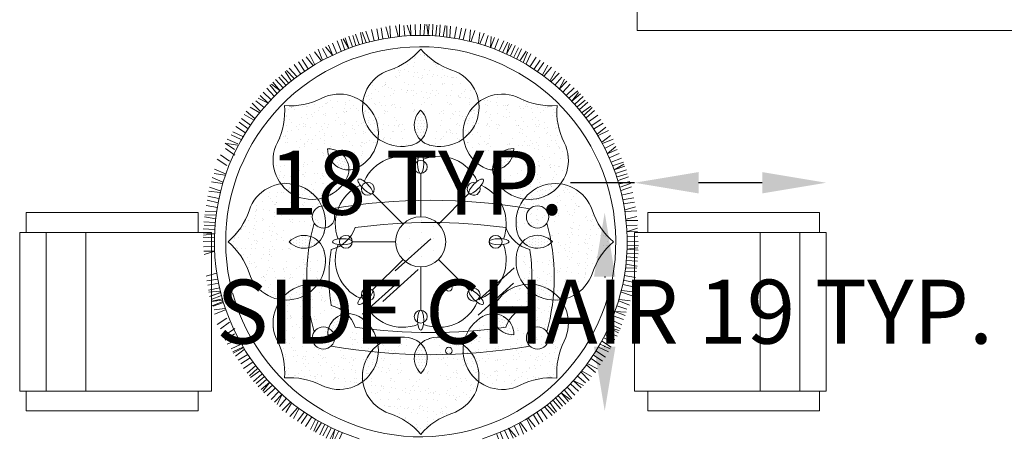
# Model space of a CAD drawing. Units: inches. Extents: x 1994 to 3075, y 3517 to 3950.
# Tile 56 of 58: x 2927 to 3019, y 3698 to 3737. Entities that reach past the tile are written whole.
import ezdxf

# ---------------------------------------------------------------- set-up
doc = ezdxf.new("R2010")
doc.units = ezdxf.units.IN
for name, color, linetype, lineweight in [('A-ANNO-DIMS', 2, 'Continuous', 18), ('A-FLOR-CASE', 8, 'Continuous', 18), ('A-FURN', 8, 'Continuous', 18), ('A-FURN-PATT', 8, 'Continuous', 13)]:
    doc.layers.add(name, color=color, linetype=linetype, lineweight=lineweight)
doc.styles.get("Standard").update_dxf_attribs({"font": 'arial.ttf'})
doc.dimstyles.get("Standard").update_dxf_attribs({"dimtxt": 6, "dimasz": 6, "dimexe": 0.18, "dimexo": 0.0625, "dimgap": 0.09, "dimtad": 0, "dimtih": 1, "dimtoh": 1, "dimdec": 4, "dimzin": 0, "dimdsep": 46, "dimlunit": 4, "dimtxsty": 'Standard', "dimcen": 0.09, "dimse1": 1, "dimse2": 1, "dimadec": 0, "dimazin": 0, "dimtfac": 1, "dimtdec": 4, "dimtofl": 0, "dimtmove": 0, "dimatfit": 3, "dimfxl": 1, "dimtolj": 1, "dimtzin": 0, "dimarcsym": 0})

# ---------------------------------------------------------------- blocks, each defined once
blk = doc.blocks.new('CHAIR-SIDE')
for p, q in [((0.619, 18.584), (16.725, 18.584)), ((0.619, 16.725), (0.619, 18.584)), ((16.725, 18.584), (16.725, 16.725)), ((0, 1.858), (0, 16.725)), ((0, 16.725), (17.964, 16.725)), ((2.478, 1.858), (2.478, 16.725)), ((6.195, 16.725), (6.195, 1.858)), ((17.964, 16.725), (17.964, 1.858)), ((17.964, 1.858), (0, 1.858)), ((0.619, 0), (0.619, 1.858)), ((16.725, 1.858), (16.725, 0)), ((16.725, 0), (0.619, 0))]:
    blk.add_line(p, q)
blk = doc.blocks.new('*D27')
at = {"layer": 'A-ANNO-DIMS', "color": 0, "lineweight": -2, "transparency": 16777216}
for p, q in [((2981.575, 3712.965), (2981.575, 3712.865)), ((2981.575, 3706.381), (2981.575, 3706.481))]:
    blk.add_line(p, q, dxfattribs=at)
at = {"layer": 'A-ANNO-DIMS', "color": 0, "transparency": 16777216}
for points in [[(2980.575, 3712.965), (2982.575, 3712.965), (2981.575, 3718.965)], [(2980.575, 3706.381), (2982.575, 3706.381), (2981.575, 3700.381)]]:
    blk.add_solid(points, dxfattribs=at)
at = {"layer": 'Defpoints', "color": 0, "transparency": 16777216}
for p in [(2984.363, 3718.965), (2981.575, 3700.381), (2984.363, 3700.381)]:
    blk.add_point(p, dxfattribs=at)
at = {"layer": 'A-ANNO-DIMS', "color": 0, "transparency": 16777216, "insert": (2981.575, 3709.673), "char_height": 6, "attachment_point": 5}
blk.add_mtext('\\A1;SIDE CHAIR 19 TYP.', dxfattribs=at)
blk = doc.blocks.new('*D28')
at = {"layer": 'A-ANNO-DIMS', "color": 0, "lineweight": -2, "transparency": 16777216}
for p, q in [((2984.363, 3721.752), (2978.363, 3721.752)), ((2996.327, 3721.752), (2990.363, 3721.752))]:
    blk.add_line(p, q, dxfattribs=at)
at = {"layer": 'A-ANNO-DIMS', "color": 0, "transparency": 16777216}
for points in [[(2990.363, 3722.752), (2990.363, 3720.752), (2984.363, 3721.752)], [(2996.327, 3722.752), (2996.327, 3720.752), (3002.327, 3721.752)]]:
    blk.add_solid(points, dxfattribs=at)
at = {"layer": 'Defpoints', "color": 0, "transparency": 16777216}
for p in [(2984.363, 3721.752), (2984.363, 3718.965), (3002.327, 3718.965)]:
    blk.add_point(p, dxfattribs=at)
at = {"layer": 'A-ANNO-DIMS', "color": 0, "transparency": 16777216, "insert": (2963.952, 3721.752), "char_height": 6, "attachment_point": 5}
blk.add_mtext('\\A1;18 TYP.', dxfattribs=at)

msp = doc.modelspace()

# ---------------------------------------------------------------- hatches: boundary and pattern name
at = {"layer": 'A-FURN-PATT'}
h = msp.add_hatch(dxfattribs=at)
h.set_pattern_fill('AR-SAND', color=256, scale=0.026605, angle=360, style=0)
h.set_pattern_definition([(142.5, (5370.1894, -656.1987), (0.04256891, 1.30208636), [0, -1.02716777, 0, -1.14880606, 0, -1.09812344]), (172.5, (5370.1894, -656.1987), (-1.19595894, 1.90711676), [0, -0.55412998, 0, -0.92580253, 0, -0.35477834]), (212.5, (5371.0206, -656.1987), (-2.10443915, 0.00382364), [0, -0.33788413, 0, -1.21638288, 0, -1.58805543]), (222.5, (5371.0206, -656.1987), (-2.03144575, 0.5931046), [0, -0.16894207, 0, -0.79740656, 0, -0.91228716])])
edge = h.paths.add_edge_path()
edge.add_arc((2962.5504, 3728.8135), 3.6655, 107.812699, 285.649719)
edge.add_arc((2959.3618, 3738.5104), 6.5423, 288.420626, 319.620203)
edge.add_arc((2969.2772, 3738.4234), 6.4463, 220.090626, 251.693416)
edge.add_arc((2966.1342, 3728.8126), 3.6654, 254.29987, 432.237712)
edge.add_arc((2963.0189, 3727.1423), 1.9224, 284.388921, 407.042497)
edge.add_arc((2965.6739, 3727.1548), 1.9373, 133.962849, 255.378029)
h = msp.add_hatch(dxfattribs=at)
h.set_pattern_fill('AR-SAND', color=256, scale=0.026605, angle=315, style=0)
h.set_pattern_definition([(187.5, (7757.3008, 2325.6455), (-0.89061333, 0.95081486), [0, -1.02716777, 0, -1.14880606, 0, -1.09812344]), (217.5, (7757.3008, 2325.6455), (-2.19420587, 0.5028645), [0, -0.55412998, 0, -0.92580253, 0, -0.35477834]), (257.5, (7757.8886, 2326.2333), (-1.49076691, -1.48535947), [0, -0.33788413, 0, -1.21638288, 0, -1.58805543]), (267.5, (7757.8886, 2326.2333), (-1.85583734, -1.0170608), [0, -0.16894207, 0, -0.79740656, 0, -0.91228716])])
edge = h.paths.add_edge_path()
edge.add_arc((2954.1711, 3723.8596), 3.6655, 152.812698, 330.649719)
edge.add_arc((2945.0597, 3728.4616), 6.5423, 333.420626, 364.620203)
edge.add_arc((2952.1325, 3735.4113), 6.4463, 265.090626, 296.693416)
edge.add_arc((2956.7059, 3726.393), 3.6654, 299.29987, 477.237712)
edge.add_arc((2955.6841, 3723.0091), 1.9224, 329.388921, 452.042497)
edge.add_arc((2957.5527, 3724.8953), 1.9373, 178.962849, 300.378029)
h = msp.add_hatch(dxfattribs=at)
h.set_pattern_fill('AR-SAND', color=256, scale=0.026605, angle=405, style=0)
h.set_pattern_definition([(97.5, (1573.7644, -1076.7382), (0.95081486, 0.89061333), [0, -1.02716777, 0, -1.14880606, 0, -1.09812344]), (127.5, (1573.7644, -1076.7382), (0.5028645, 2.19420587), [0, -0.55412998, 0, -0.92580253, 0, -0.35477834]), (167.5, (1574.3522, -1077.326), (-1.48535947, 1.49076691), [0, -0.33788413, 0, -1.21638288, 0, -1.58805543]), (177.5, (1574.3522, -1077.326), (-1.0170608, 1.85583734), [0, -0.16894207, 0, -0.79740656, 0, -0.91228716])])
edge = h.paths.add_edge_path()
edge.add_arc((2971.9785, 3726.3915), 3.6655, 62.812699, 240.649719)
edge.add_arc((2976.5805, 3735.5029), 6.5423, 243.420626, 274.620203)
edge.add_arc((2983.5302, 3728.4301), 6.4463, 175.090626, 206.693416)
edge.add_arc((2974.5119, 3723.8567), 3.6654, 209.29987, 387.237712)
edge.add_arc((2971.128, 3724.8785), 1.9224, 239.388921, 362.042497)
edge.add_arc((2973.0142, 3723.0099), 1.9373, 88.962849, 210.378029)
h = msp.add_hatch(dxfattribs=at)
h.set_pattern_fill('DOTS', color=256, scale=0.177367, angle=360, style=0)
h.set_pattern_definition([(180, (5370.18936, -656.19867), (-0.140785056, 0.281570112), [0, -0.281570112])])
h.paths.add_polyline_path([(2964.3422, 3725.7478, 0.432463), (2964.329, 3728.5493, 0.4276325)])
h = msp.add_hatch(dxfattribs=at)
h.set_pattern_fill('DOTS', color=256, scale=0.177367, angle=315, style=0)
h.set_pattern_definition([(225, (7757.30082, 2325.64553), (-0.298650203, 0.099550068), [0, -0.281570112])])
h.paths.add_polyline_path([(2957.6059, 3722.9587, 0.432463), (2955.6156, 3724.9304, 0.4276325)])
h = msp.add_hatch(dxfattribs=at)
h.set_pattern_fill('DOTS', color=256, scale=0.177367, angle=405, style=0)
h.set_pattern_definition([(135, (1573.76442, -1076.73822), (0.099550068, 0.298650203), [0, -0.281570112])])
h.paths.add_polyline_path([(2971.0776, 3722.9567, 0.432463), (2973.0492, 3724.947, 0.4276325)])
h = msp.add_hatch(dxfattribs=at)
h.set_pattern_fill('AR-SAND', color=256, scale=0.026605, angle=630, style=0)
h.set_pattern_definition([(232.5, (7336.7613, 6122.0705), (-1.30208636, 0.04256891), [0, -1.02716777, 0, -1.14880606, 0, -1.09812344]), (262.5, (7336.7613, 6122.0705), (-1.90711676, -1.19595894), [0, -0.55412998, 0, -0.92580253, 0, -0.35477834]), (302.5, (7336.7613, 6122.9017), (-0.00382364, -2.10443915), [0, -0.33788413, 0, -1.21638288, 0, -1.58805543]), (312.5, (7336.7613, 6122.9017), (-0.5931046, -2.03144575), [0, -0.16894207, 0, -0.79740656, 0, -0.91228716])])
edge = h.paths.add_edge_path()
edge.add_arc((2951.7491, 3714.4315), 3.6655, 197.812698, 375.649719)
edge.add_arc((2942.0522, 3711.2429), 6.5423, 18.420626, 49.620203)
edge.add_arc((2942.1392, 3721.1583), 6.4463, 310.090626, 341.693416)
edge.add_arc((2951.75, 3718.0153), 3.6654, 344.29987, 522.237712)
edge.add_arc((2953.4203, 3714.9001), 1.9224, 14.388921, 137.042497)
edge.add_arc((2953.4078, 3717.555), 1.9373, 223.962849, 345.378029)
h = msp.add_hatch(dxfattribs=at)
h.set_pattern_fill('AR-SAND', color=256, scale=0.026605, angle=450, style=0)
h.set_pattern_definition([(52.5, (-1408.0798, 1310.3732), (1.30208636, -0.04256891), [0, -1.02716777, 0, -1.14880606, 0, -1.09812344]), (82.5, (-1408.0798, 1310.3732), (1.90711676, 1.19595894), [0, -0.55412998, 0, -0.92580253, 0, -0.35477834]), (122.5, (-1408.0798, 1309.542), (0.00382364, 2.10443915), [0, -0.33788413, 0, -1.21638288, 0, -1.58805543]), (132.5, (-1408.0798, 1309.542), (0.5931046, 2.03144575), [0, -0.16894207, 0, -0.79740656, 0, -0.91228716])])
edge = h.paths.add_edge_path()
edge.add_arc((2976.9324, 3718.0122), 3.6655, 17.812698, 195.649719)
edge.add_arc((2986.6293, 3721.2008), 6.5423, 198.420626, 229.620203)
edge.add_arc((2986.5423, 3711.2854), 6.4463, 130.090626, 161.693416)
edge.add_arc((2976.9315, 3714.4285), 3.6654, 164.29987, 342.237712)
edge.add_arc((2975.2612, 3717.5437), 1.9224, 194.388921, 317.042497)
edge.add_arc((2975.2737, 3714.8887), 1.9373, 43.962849, 165.378029)
h = msp.add_hatch(dxfattribs=at)
h.set_pattern_fill('DOTS', color=256, scale=17.7367, angle=450, style=0)
h.set_pattern_definition([(90, (2796.9945, 3617.8875), (1.108544, 0.554272), [0, -1.108544])])
h.paths.add_polyline_path([(2964.3407, 3718.5711, 1), (2964.3407, 3713.8726, 1)])
h = msp.add_hatch(dxfattribs=at)
h.set_pattern_fill('DOTS', color=256, scale=0.177367, angle=630, style=0)
h.set_pattern_definition([(270, (7336.76127, 6122.07047), (-0.281570112, -0.140785056), [0, -0.281570112])])
h.paths.add_polyline_path([(2954.8149, 3716.2233, 0.432463), (2952.0133, 3716.2101, 0.4276325)])
h = msp.add_hatch(dxfattribs=at)
h.set_pattern_fill('DOTS', color=256, scale=0.177367, angle=450, style=0)
h.set_pattern_definition([(90, (-1408.07978, 1310.37324), (0.281570112, 0.140785056), [0, -0.281570112])])
h.paths.add_polyline_path([(2973.8666, 3716.2204, 0.432463), (2976.6682, 3716.2336, 0.4276325)])
h = msp.add_hatch(dxfattribs=at)
h.set_pattern_fill('AR-SAND', color=256, scale=0.026605, angle=585, style=0)
h.set_pattern_definition([(277.5, (4354.9171, 8509.1819), (-0.95081486, -0.89061333), [0, -1.02716777, 0, -1.14880606, 0, -1.09812344]), (307.5, (4354.917, 8509.182), (-0.5028645, -2.19420587), [0, -0.55412998, 0, -0.92580253, 0, -0.35477834]), (347.5, (4354.3293, 8509.7697), (1.48535947, -1.49076691), [0, -0.33788413, 0, -1.21638288, 0, -1.58805543]), (357.5, (4354.3293, 8509.7697), (1.0170608, -1.85583734), [0, -0.16894207, 0, -0.79740656, 0, -0.91228716])])
edge = h.paths.add_edge_path()
edge.add_arc((2956.703, 3706.0522), 3.6655, 242.812699, 420.649719)
edge.add_arc((2952.101, 3696.9408), 6.5423, 63.420626, 94.620203)
edge.add_arc((2945.1513, 3704.0136), 6.4463, 355.090626, 386.693416)
edge.add_arc((2954.1696, 3708.587), 3.6654, 29.29987, 207.237712)
edge.add_arc((2957.5535, 3707.5653), 1.9224, 59.388921, 182.042497)
edge.add_arc((2955.6673, 3709.4338), 1.9373, 268.962849, 390.378029)
h = msp.add_hatch(dxfattribs=at)
h.set_pattern_fill('AR-SAND', color=256, scale=0.026605, angle=495, style=0)
h.set_pattern_definition([(7.5, (-1828.6193, 5106.7982), (0.89061333, -0.95081486), [0, -1.02716777, 0, -1.14880606, 0, -1.09812344]), (37.5, (-1828.6193, 5106.7982), (2.19420587, -0.5028645), [0, -0.55412998, 0, -0.92580253, 0, -0.35477834]), (77.5, (-1829.2071, 5106.2104), (1.49076691, 1.48535947), [0, -0.33788413, 0, -1.21638288, 0, -1.58805543]), (87.5, (-1829.207, 5106.2104), (1.85583734, 1.0170608), [0, -0.16894207, 0, -0.79740656, 0, -0.91228716])])
edge = h.paths.add_edge_path()
edge.add_arc((2974.5104, 3708.5841), 3.6655, 332.812698, 510.649719)
edge.add_arc((2983.6218, 3703.9821), 6.5423, 153.420626, 184.620203)
edge.add_arc((2976.549, 3697.0324), 6.4463, 85.090626, 116.693416)
edge.add_arc((2971.9756, 3706.0507), 3.6654, 119.29987, 297.237712)
edge.add_arc((2972.9973, 3709.4346), 1.9224, 149.388921, 272.042497)
edge.add_arc((2971.1288, 3707.5484), 1.9373, 358.962849, 480.378029)
h = msp.add_hatch(dxfattribs=at)
h.set_pattern_fill('DOTS', color=256, scale=0.177367, angle=585, style=0)
h.set_pattern_definition([(315, (4354.91707, 8509.18193), (-0.099550068, -0.298650203), [0, -0.281570112])])
h.paths.add_polyline_path([(2957.6039, 3709.487, 0.432463), (2955.6322, 3707.4967, 0.4276325)])
h = msp.add_hatch(dxfattribs=at)
h.set_pattern_fill('DOTS', color=256, scale=0.177367, angle=495, style=0)
h.set_pattern_definition([(45, (-1828.61933, 5106.79818), (0.298650203, -0.099550068), [0, -0.281570112])])
h.paths.add_polyline_path([(2971.0756, 3709.485, 0.432463), (2973.0659, 3707.5134, 0.4276325)])
h = msp.add_hatch(dxfattribs=at)
h.set_pattern_fill('AR-SAND', color=256, scale=0.026605, angle=540, style=0)
h.set_pattern_definition([(322.5, (558.4921, 8088.6424), (-0.04256891, -1.30208636), [0, -1.02716777, 0, -1.14880606, 0, -1.09812344]), (352.5, (558.4921, 8088.6424), (1.19595894, -1.90711676), [0, -0.55412998, 0, -0.92580253, 0, -0.35477834]), (32.5, (557.6609, 8088.6424), (2.10443915, -0.00382364), [0, -0.33788413, 0, -1.21638288, 0, -1.58805543]), (42.5, (557.661, 8088.6424), (2.03144575, -0.5931046), [0, -0.16894207, 0, -0.79740656, 0, -0.91228716])])
edge = h.paths.add_edge_path()
edge.add_arc((2966.1311, 3703.6302), 3.6655, 287.812699, 465.649719)
edge.add_arc((2969.3197, 3693.9333), 6.5423, 108.420626, 139.620203)
edge.add_arc((2959.4043, 3694.0203), 6.4463, 40.090626, 71.693416)
edge.add_arc((2962.5473, 3703.6311), 3.6654, 74.29987, 252.237712)
edge.add_arc((2965.6625, 3705.3014), 1.9224, 104.388921, 227.042497)
edge.add_arc((2963.0076, 3705.2889), 1.9373, 313.962849, 435.378029)
h = msp.add_hatch(dxfattribs=at)
h.set_pattern_fill('DOTS', color=256, scale=0.177367, angle=540, style=0)
h.set_pattern_definition([(360, (558.49213, 8088.64238), (0.140785056, -0.281570112), [0, -0.281570112])])
h.paths.add_polyline_path([(2964.3393, 3706.696, 0.432463), (2964.3525, 3703.8944, 0.4276325)])

# ---------------------------------------------------------------- linework, layer by layer
at = {"layer": 'A-FLOR-CASE'}
for p, q in [((2984.6205, 3755.1269), (2984.6205, 3736.0298)), ((2984.6205, 3736.0298), (3024.072, 3736.0298))]:
    msp.add_line(p, q, dxfattribs=at)
at = {"layer": 'A-FURN'}
for p, q in [((2961.5141, 3735.3945), (2961.4302, 3736.4562)), ((2962.2132, 3735.4783), (2961.9615, 3736.4562)), ((2962.353, 3735.4783), (2962.353, 3736.568)), ((2962.8564, 3735.4783), (2962.7725, 3736.4841)), ((2963.4157, 3735.5062), (2963.0801, 3736.5121)), ((2963.3877, 3736.54), (2963.4157, 3735.5062)), ((2963.8072, 3736.568), (2963.8352, 3735.5342)), ((2964.3106, 3736.5959), (2964.2826, 3735.5621)), ((2964.73, 3736.6238), (2964.6461, 3735.5342)), ((2965.0377, 3735.5342), (2964.8978, 3736.568)), ((2965.1215, 3736.5959), (2965.0377, 3735.5342)), ((2965.4851, 3736.5959), (2965.4292, 3735.5342)), ((2965.8486, 3736.5121), (2965.7647, 3735.5342)), ((2966.1003, 3735.5062), (2966.1562, 3736.54)), ((2966.4359, 3735.4224), (2966.6316, 3736.4841)), ((2966.7715, 3735.4224), (2966.7994, 3736.4562)), ((2967.0791, 3735.3945), (2967.135, 3736.4282)), ((2957.6012, 3735.4829), (2957.9558, 3734.4806)), ((2957.9691, 3735.5446), (2958.2658, 3734.6091)), ((2958.5866, 3734.7117), (2958.2426, 3735.6881)), ((2958.9287, 3734.7626), (2958.7032, 3735.8184)), ((2959.2387, 3734.8911), (2958.8689, 3735.8568)), ((2959.5336, 3734.983), (2959.1897, 3735.9594)), ((2959.9639, 3735.0402), (2959.7385, 3736.096)), ((2960.4094, 3735.134), (2960.2204, 3736.1747)), ((2960.787, 3735.2268), (2960.6192, 3736.2606)), ((2961.3463, 3735.3665), (2961.0666, 3736.3444)), ((2967.4986, 3735.2827), (2967.6943, 3736.3444)), ((2967.946, 3735.1989), (2968.1697, 3736.2327)), ((2968.3304, 3735.1401), (2968.571, 3736.1594)), ((2968.9006, 3735.0552), (2969.0164, 3736.0656)), ((2969.0663, 3735.0168), (2969.3951, 3736.0298)), ((2969.7443, 3734.8267), (2969.886, 3735.8264)), ((2969.8735, 3734.7732), (2970.2905, 3735.7799)), ((2970.3385, 3734.5805), (2970.6459, 3735.5419)), ((2970.8659, 3734.3923), (2970.9408, 3735.45)), ((2955.6849, 3734.6287), (2956.1063, 3733.6843)), ((2956.0617, 3734.815), (2956.4831, 3733.8706)), ((2956.5161, 3735.0335), (2956.8858, 3734.0677)), ((2956.8929, 3735.2198), (2957.2324, 3734.181)), ((2957.5941, 3734.3308), (2957.0693, 3735.2324)), ((2957.2653, 3735.3438), (2957.5941, 3734.3308)), ((2971.2357, 3735.3581), (2970.8659, 3734.3923)), ((2971.6339, 3735.2234), (2971.2642, 3734.2576)), ((2972.1097, 3735.0566), (2971.6882, 3734.1122)), ((2972.5079, 3734.9218), (2972.0134, 3733.9472)), ((2972.3751, 3733.7974), (2972.6415, 3734.806)), ((2972.8589, 3734.7462), (2972.3751, 3733.7974)), ((2973.1948, 3734.6071), (2972.7368, 3733.6476)), ((2954.3922, 3732.8533), (2953.9084, 3733.8021)), ((2955.006, 3733.1983), (2954.3993, 3734.0055)), ((2955.1352, 3733.2518), (2954.7182, 3734.2585)), ((2955.6003, 3733.4445), (2955.1378, 3734.3416)), ((2956.1063, 3733.6843), (2955.4113, 3734.4851)), ((2973.4986, 3734.3905), (2973.0468, 3733.5192)), ((2973.3462, 3733.3649), (2973.7935, 3734.2986)), ((2973.6241, 3733.1591), (2974.2113, 3734.0651)), ((2973.9342, 3733.0307), (2974.3556, 3733.975)), ((2974.2077, 3732.8871), (2974.655, 3733.8208)), ((2953.0956, 3731.9328), (2952.4833, 3732.822)), ((2953.4712, 3732.1899), (2952.8985, 3733.0791)), ((2953.7846, 3732.4202), (2953.234, 3733.3111)), ((2954.2479, 3732.7633), (2953.6153, 3733.5597)), ((2974.5525, 3732.6234), (2975.1396, 3733.5293)), ((2974.9338, 3732.3747), (2975.5361, 3733.2442)), ((2975.2664, 3732.1733), (2975.8788, 3733.0229)), ((2975.7607, 3731.8766), (2976.2544, 3732.7658)), ((2951.9488, 3731.1022), (2951.2574, 3731.8727)), ((2952.2454, 3731.2802), (2951.6331, 3732.1694)), ((2952.4827, 3731.5175), (2951.7715, 3732.2682)), ((2952.7199, 3731.7152), (2952.0285, 3732.4858)), ((2975.8991, 3731.7777), (2976.5905, 3732.5878)), ((2976.4527, 3731.3426), (2976.9662, 3732.2121)), ((2976.5516, 3731.2437), (2977.3221, 3732.0142)), ((2950.1896, 3730.9235), (2950.9008, 3730.0937)), ((2951.1777, 3730.3705), (2950.3478, 3731.0026)), ((2950.4862, 3731.1806), (2951.1777, 3730.3705)), ((2950.7433, 3731.4376), (2951.4545, 3730.6474)), ((2951.0596, 3731.6354), (2951.6918, 3730.8846)), ((2976.9075, 3730.8878), (2977.5594, 3731.6584)), ((2977.3228, 3730.5121), (2977.7967, 3731.4606)), ((2978.034, 3731.2628), (2977.3228, 3730.5121)), ((2978.3503, 3730.986), (2977.6391, 3730.2352)), ((2949.2998, 3729.9151), (2950.0505, 3729.2039)), ((2949.5766, 3730.2314), (2950.3274, 3729.5202)), ((2949.9128, 3730.6071), (2950.624, 3729.8564)), ((2978.726, 3730.6498), (2977.9753, 3729.9386)), ((2979.0424, 3730.373), (2978.2126, 3729.6618)), ((2978.4894, 3729.3849), (2979.1215, 3730.2148)), ((2979.2995, 3730.0764), (2978.4894, 3729.3849)), ((2949.3189, 3728.4327), (2948.5484, 3729.2032)), ((2949.6748, 3728.7886), (2948.9042, 3729.4405)), ((2950.0505, 3729.2039), (2949.102, 3729.6778)), ((2979.5565, 3729.8193), (2978.7662, 3729.1081)), ((2979.7543, 3729.503), (2979.0035, 3728.8708)), ((2979.2211, 3728.6138), (2979.9916, 3729.3052)), ((2948.686, 3727.6418), (2947.7968, 3728.1355)), ((2948.7849, 3727.7802), (2947.9748, 3728.4716)), ((2949.22, 3728.3338), (2948.3505, 3728.8473)), ((2979.3991, 3728.3172), (2980.2882, 3728.9295)), ((2979.6364, 3728.0799), (2980.3871, 3728.7911)), ((2979.8341, 3727.8427), (2980.6047, 3728.5341)), ((2980.0517, 3727.467), (2980.9409, 3728.0793)), ((2948.1879, 3726.8149), (2947.3184, 3727.4172)), ((2948.3893, 3727.1475), (2947.5397, 3727.7599)), ((2980.3088, 3727.0914), (2981.198, 3727.6642)), ((2980.5391, 3726.778), (2981.43, 3727.3286)), ((2947.5319, 3725.8153), (2946.5876, 3726.2367)), ((2947.6755, 3726.0888), (2946.7418, 3726.5361)), ((2947.9392, 3726.4336), (2947.0333, 3727.0207)), ((2980.8822, 3726.3147), (2981.6786, 3726.9473)), ((2980.9722, 3726.1704), (2981.921, 3726.6542)), ((2946.8904, 3724.8519), (2946.0209, 3725.4542)), ((2947.1615, 3725.2774), (2946.1617, 3725.4191)), ((2947.215, 3725.4065), (2946.2083, 3725.8235)), ((2981.3172, 3725.5566), (2982.1243, 3726.1633)), ((2981.3707, 3725.4274), (2982.3774, 3725.8444)), ((2981.5633, 3724.9623), (2982.4605, 3725.4248)), ((2946.9107, 3724.3389), (2946.0611, 3724.9513)), ((2981.8032, 3724.4563), (2982.604, 3725.1513)), ((2982.7476, 3724.8778), (2981.8032, 3724.4563)), ((2982.9339, 3724.5009), (2981.9895, 3724.0795)), ((2946.1891, 3723.3833), (2945.2831, 3723.9705)), ((2946.4377, 3723.7647), (2945.5683, 3724.3669)), ((2983.1523, 3724.0465), (2982.1866, 3723.6768)), ((2983.3387, 3723.6697), (2982.2999, 3723.3302)), ((2982.4497, 3722.9685), (2983.3513, 3723.4933)), ((2945.9846, 3722.4687), (2944.9848, 3722.6104)), ((2946.0381, 3722.5979), (2945.0314, 3723.0149)), ((2964.3407, 3718.5711), (2964.3407, 3722.5992)), ((2983.4627, 3723.2973), (2982.4497, 3722.9685)), ((2983.6018, 3722.9614), (2982.5995, 3722.6068)), ((2983.6635, 3722.5935), (2982.7279, 3722.2968)), ((2945.7432, 3721.6835), (2944.7434, 3721.8252)), ((2945.7967, 3721.8127), (2944.79, 3722.2297)), ((2982.8306, 3721.976), (2983.807, 3722.32)), ((2982.8815, 3721.6339), (2983.9373, 3721.8594)), ((2983.01, 3721.3239), (2983.9757, 3721.6937)), ((2945.5147, 3720.8399), (2944.5042, 3720.9557)), ((2945.5531, 3721.0056), (2944.5401, 3721.3343)), ((2962.6796, 3717.883), (2959.8313, 3720.7313)), ((2966.0019, 3717.883), (2968.8502, 3720.7313)), ((2983.1019, 3721.029), (2984.0783, 3721.3729)), ((2983.1591, 3720.5987), (2984.2149, 3720.8241)), ((2945.371, 3719.8852), (2944.3372, 3720.109)), ((2945.4297, 3720.2697), (2944.4104, 3720.5103)), ((2983.2529, 3720.1532), (2984.2936, 3720.3422)), ((2983.3457, 3719.7756), (2984.3795, 3719.9434)), ((2945.1754, 3719.0183), (2944.1416, 3719.0743)), ((2945.2871, 3719.4378), (2944.2254, 3719.6336)), ((2983.4854, 3719.2163), (2984.4633, 3719.496)), ((2983.5134, 3719.0485), (2984.5751, 3719.1324)), ((2945.0636, 3718.0396), (2944.0299, 3718.0955)), ((2945.1474, 3718.3751), (2944.0857, 3718.5709)), ((2945.1474, 3718.7107), (2944.1137, 3718.7387)), ((2983.5972, 3718.3494), (2984.5751, 3718.6011)), ((2983.5972, 3718.2096), (2984.6868, 3718.2096)), ((2943.974, 3717.4243), (2945.0357, 3717.3684)), ((2943.974, 3717.0608), (2945.0357, 3716.9769)), ((2944.0578, 3717.7879), (2945.0357, 3717.704)), ((2983.5972, 3717.7062), (2984.603, 3717.7901)), ((2983.6251, 3717.1469), (2984.631, 3717.4825)), ((2984.6589, 3717.1749), (2983.6251, 3717.1469)), ((2943.946, 3716.6693), (2945.0357, 3716.5854)), ((2943.974, 3716.2498), (2945.0077, 3716.2219)), ((2945.0357, 3716.9769), (2944.0019, 3716.8371)), ((2961.9915, 3716.2219), (2957.9634, 3716.2219)), ((2965.2735, 3716.4984), (2961.9543, 3713.4973)), ((2984.6868, 3716.7554), (2983.6531, 3716.7274)), ((2984.7148, 3716.252), (2983.681, 3716.28)), ((2944.0019, 3715.7464), (2945.0357, 3715.7744)), ((2944.0299, 3715.327), (2945.0636, 3715.355)), ((2945.0636, 3715.355), (2944.0578, 3715.0194)), ((2984.7427, 3715.8326), (2983.6531, 3715.9165)), ((2983.6531, 3715.525), (2984.6868, 3715.6648)), ((2984.7148, 3715.4411), (2983.6531, 3715.525)), ((2962.6796, 3714.5607), (2959.8313, 3711.7124)), ((2966.0019, 3714.5607), (2968.8502, 3711.7124)), ((2983.6251, 3714.4623), (2984.6589, 3714.4064)), ((2984.7148, 3715.0775), (2983.6531, 3715.1334)), ((2984.631, 3714.714), (2983.6531, 3714.7979)), ((2964.1135, 3713.6145), (2960.7943, 3710.6135)), ((2964.3407, 3713.8726), (2964.3407, 3709.8445)), ((2973.0926, 3713.7736), (2969.7734, 3710.7726)), ((2983.5134, 3713.4835), (2984.5471, 3713.4276)), ((2983.5413, 3714.1267), (2984.603, 3713.931)), ((2983.5413, 3713.7911), (2984.5751, 3713.7632)), ((2945.2033, 3713.2856), (2944.2254, 3713.0059)), ((2945.343, 3712.7263), (2944.3093, 3712.5585)), ((2962.2169, 3712.4299), (2958.8977, 3709.4289)), ((2983.3178, 3712.6166), (2984.3516, 3712.3929)), ((2983.4016, 3713.064), (2984.4633, 3712.8683)), ((2945.4358, 3712.3486), (2944.3951, 3712.1597)), ((2945.5296, 3711.9032), (2944.4738, 3711.6777)), ((2945.5147, 3711.6039), (2944.5042, 3711.488)), ((2945.5869, 3711.4728), (2944.6104, 3711.1289)), ((2973.0436, 3712.3509), (2969.7245, 3709.3499)), ((2983.1357, 3711.4963), (2984.1487, 3711.1675)), ((2983.1741, 3711.662), (2984.1845, 3711.5462)), ((2983.259, 3712.2322), (2984.2783, 3711.9916)), ((2945.5531, 3711.4382), (2944.5401, 3711.1094)), ((2945.6788, 3711.178), (2944.713, 3710.8082)), ((2945.7432, 3710.7602), (2944.7434, 3710.6185)), ((2945.8072, 3710.8679), (2944.7514, 3710.6425)), ((2945.7967, 3710.631), (2944.79, 3710.214)), ((2982.892, 3710.6891), (2983.8988, 3710.2722)), ((2982.9456, 3710.8183), (2983.9453, 3710.6766)), ((2945.8582, 3710.5258), (2944.8817, 3710.1819)), ((2945.9846, 3709.975), (2944.9848, 3709.8333)), ((2946.0381, 3709.8458), (2945.0314, 3709.4288)), ((2982.5112, 3709.6967), (2983.5689, 3709.6218)), ((2983.477, 3709.3269), (2982.5112, 3709.6967)), ((2982.6994, 3710.2241), (2983.6608, 3709.9167)), ((2946.1891, 3709.0604), (2945.2831, 3708.4732)), ((2983.1754, 3708.4529), (2982.2311, 3708.8744)), ((2983.3423, 3708.9287), (2982.3765, 3709.2984)), ((2946.4377, 3708.6791), (2945.5683, 3708.0768)), ((2946.9107, 3708.1048), (2946.0611, 3707.4925)), ((2982.726, 3707.3678), (2981.7665, 3707.8258)), ((2982.8651, 3707.7037), (2981.9163, 3708.1875)), ((2981.9163, 3708.1875), (2982.9249, 3707.9211)), ((2983.0407, 3708.0547), (2982.0661, 3708.5492)), ((2946.8904, 3707.5919), (2946.0209, 3706.9896)), ((2947.1615, 3707.1664), (2946.1617, 3707.0247)), ((2947.215, 3707.0372), (2946.2083, 3706.6202)), ((2981.278, 3706.9385), (2982.184, 3706.3513)), ((2981.4838, 3707.2164), (2982.4175, 3706.7691)), ((2982.5094, 3707.064), (2981.6381, 3707.5158)), ((2947.5319, 3706.6284), (2946.5876, 3706.207)), ((2947.6755, 3706.3549), (2946.7418, 3705.9076)), ((2947.7093, 3706.2733), (2946.7605, 3705.7895)), ((2947.7993, 3706.129), (2947.0029, 3705.4964)), ((2980.7422, 3706.0101), (2981.6482, 3705.423)), ((2981.006, 3706.3549), (2981.9397, 3705.9076)), ((2981.1496, 3706.6284), (2982.0939, 3706.207)), ((2948.1424, 3705.6657), (2947.2515, 3705.1151)), ((2948.3727, 3705.3523), (2947.4835, 3704.7796)), ((2980.2922, 3705.2962), (2981.1418, 3704.6838)), ((2980.4936, 3705.6288), (2981.363, 3705.0265)), ((2948.6298, 3704.9767), (2947.7406, 3704.3644)), ((2948.8474, 3704.601), (2948.0768, 3703.9096)), ((2949.0451, 3704.3638), (2948.2944, 3703.6526)), ((2949.2824, 3704.1265), (2948.3933, 3703.5142)), ((2979.4615, 3704.1099), (2980.331, 3703.5964)), ((2979.8966, 3704.6635), (2980.7067, 3703.9721)), ((2979.9955, 3704.8019), (2980.8847, 3704.3082)), ((2949.4604, 3703.8299), (2948.6899, 3703.1385)), ((2948.9272, 3702.9407), (2949.678, 3703.5729)), ((2949.125, 3702.6244), (2949.9152, 3703.3356)), ((2978.631, 3703.2398), (2979.5795, 3702.7659)), ((2979.3817, 3702.5286), (2978.631, 3703.2398)), ((2979.0067, 3703.6551), (2979.7773, 3703.0032)), ((2979.3626, 3704.011), (2980.1331, 3703.2405)), ((2949.382, 3702.3674), (2950.1921, 3703.0588)), ((2950.1921, 3703.0588), (2949.56, 3702.2289)), ((2949.6391, 3702.0708), (2950.4689, 3702.7819)), ((2949.9555, 3701.7939), (2950.7062, 3702.5051)), ((2978.4919, 3701.5202), (2977.7807, 3702.35)), ((2978.7687, 3701.8366), (2978.0575, 3702.5873)), ((2979.1049, 3702.2123), (2978.3541, 3702.9235)), ((2950.3312, 3701.4577), (2951.0424, 3702.2085)), ((2950.6475, 3701.1809), (2951.3587, 3701.9316)), ((2951.3587, 3701.9316), (2950.8848, 3700.9831)), ((2951.774, 3701.5559), (2951.1221, 3700.7853)), ((2976.7327, 3701.3415), (2977.4241, 3700.571)), ((2977.6219, 3700.8083), (2976.9897, 3701.5591)), ((2977.9382, 3701.0061), (2977.227, 3701.7964)), ((2977.5038, 3702.0732), (2978.3337, 3701.4411)), ((2978.1953, 3701.2631), (2977.5038, 3702.0732)), ((2952.1299, 3701.2), (2951.3594, 3700.4295)), ((2952.2288, 3701.1011), (2951.7153, 3700.2317)), ((2952.7824, 3700.666), (2952.091, 3699.8559)), ((2952.9208, 3700.5671), (2952.4271, 3699.6779)), ((2975.5859, 3700.5109), (2976.1982, 3699.6217)), ((2975.9616, 3700.7285), (2976.653, 3699.9579)), ((2976.1988, 3700.9262), (2976.91, 3700.1755)), ((2976.4361, 3701.1635), (2977.0484, 3700.2744)), ((2953.4151, 3700.2704), (2952.8027, 3699.4208)), ((2953.7477, 3700.069), (2953.1454, 3699.1996)), ((2954.129, 3699.8204), (2953.5419, 3698.9144)), ((2954.4738, 3699.5566), (2954.0265, 3698.6229)), ((2974.2893, 3699.5904), (2974.7731, 3698.6416)), ((2974.4336, 3699.6804), (2975.0662, 3698.884)), ((2974.8969, 3700.0235), (2975.4475, 3699.1326)), ((2975.2103, 3700.2538), (2975.783, 3699.3646)), ((2954.7473, 3699.413), (2954.3259, 3698.4687)), ((2955.0573, 3699.2846), (2954.4702, 3698.3786)), ((2955.3353, 3699.0788), (2954.888, 3698.1451)), ((2955.1829, 3698.0532), (2955.6346, 3698.9245)), ((2955.4867, 3697.8366), (2955.9447, 3698.7961)), ((2955.8604, 3697.7717), (2956.3064, 3698.6463)), ((2956.3064, 3698.6463), (2956.0754, 3697.7717)), ((2972.556, 3697.7717), (2972.1983, 3698.5731)), ((2972.5752, 3698.7594), (2973.2701, 3697.9586)), ((2972.9966, 3697.815), (2972.5752, 3698.7594)), ((2973.0812, 3698.9993), (2973.5437, 3698.1021)), ((2973.5463, 3699.1919), (2973.9633, 3698.1852)), ((2973.6755, 3699.2454), (2974.2822, 3698.4383)), ((2956.3004, 3697.7717), (2956.6681, 3698.4965)), ((2956.7434, 3697.7717), (2956.9933, 3698.3315)), ((2971.6096, 3697.7717), (2971.4491, 3698.2627)), ((2972.027, 3697.7717), (2971.7957, 3698.376))]:
    msp.add_line(p, q, dxfattribs=at)
for centre, radius in [((2964.3407, 3723.2346), 0.6035), ((2959.382, 3721.1806), 0.6035), ((2955.2258, 3718.5508), 1.0433), ((2975.2811, 3718.5508), 1.0433), ((2964.3407, 3716.2219), 2.3493), ((2957.328, 3716.2219), 0.6035), ((2971.3535, 3716.2219), 0.6035), ((2959.382, 3711.2631), 0.6035), ((2966.9699, 3711.9052), 0.3155), ((2969.2995, 3711.2631), 0.6035), ((2964.3407, 3709.2091), 0.6035), ((2955.2258, 3707.2071), 1.0433), ((2975.2811, 3707.2071), 1.0433), ((2966.9699, 3706.0179), 0.3155)]:
    msp.add_circle(centre, radius, dxfattribs=at)
for centre, radius, start, end in [((2964.3407, 3716.2219), 19.333, 287.382168, 252.617838), ((2964.3407, 3716.2219), 18.2688, 195.136145, 194.666805), ((2959.3618, 3738.5104), 6.5423, 288.420626, 319.620203), ((2969.2772, 3738.4234), 6.4463, 220.090626, 251.693416), ((2962.5504, 3728.8135), 3.6655, 107.812699, 285.649719), ((2966.1342, 3728.8126), 3.6654, 254.29987, 72.237712), ((2956.7059, 3726.393), 3.6654, 299.29987, 117.237712), ((2971.9785, 3726.3915), 3.6655, 62.812699, 240.649719), ((2952.1325, 3735.4113), 6.4463, 265.090626, 296.693416), ((2976.5805, 3735.5029), 6.5423, 243.420626, 274.620203), ((2945.0597, 3728.4616), 6.5423, 333.420626, 4.620203), ((2963.0189, 3727.1423), 1.9224, 284.388921, 47.042497), ((2965.6739, 3727.1548), 1.9373, 133.962849, 255.378029), ((2983.5302, 3728.4301), 6.4463, 175.090626, 206.693416), ((2954.1711, 3723.8596), 3.6655, 152.812698, 330.649719), ((2974.5119, 3723.8567), 3.6654, 209.29987, 27.237712), ((2957.5527, 3724.8953), 1.9373, 178.962849, 300.378029), ((2955.6841, 3723.0091), 1.9224, 329.388921, 92.042497), ((2971.128, 3724.8785), 1.9224, 239.388921, 2.042497), ((2973.0142, 3723.0099), 1.9373, 88.962849, 210.378029), ((2962.6508, 3720.3017), 3.9289, 68.660791, 156.339209), ((2966.0307, 3720.3017), 3.9289, 23.660791, 111.339209), ((2951.75, 3718.0153), 3.6654, 344.29987, 162.237712), ((2969.2995, 3721.1806), 0.6035, 72.704376, 17.295624), ((2976.9324, 3718.0122), 3.6655, 17.812698, 195.649719), ((2960.2609, 3717.9118), 3.9289, 113.660791, 201.339209), ((2968.4206, 3717.9118), 3.9289, 338.660791, 66.339209), ((2965.2535, 3666.2615), 53.8543, 80.048079, 99.951921), ((2942.1392, 3721.1583), 6.4463, 310.090626, 341.693416), ((2986.6293, 3721.2008), 6.5423, 198.420626, 229.620203), ((2972.5658, 3712.8789), 18.9049, 164.377933, 195.622067), ((2965.2535, 3666.2615), 51.7676, 82.157581, 97.842419), ((2957.9412, 3712.8789), 18.9049, 344.377933, 15.622067), ((2953.4078, 3717.555), 1.9373, 223.962849, 345.378029), ((2955.2258, 3718.5508), 3.13, 283.453601, 341.255069), ((2975.2811, 3718.5508), 3.13, 198.744931, 256.546399), ((2975.2612, 3717.5437), 1.9224, 194.388921, 317.042497), ((2942.0522, 3711.2429), 6.5423, 18.420626, 49.620203), ((2953.4203, 3714.9001), 1.9224, 14.388921, 137.042497), ((2975.2737, 3714.8887), 1.9373, 43.962849, 165.378029), ((2986.5423, 3711.2854), 6.4463, 130.090626, 161.693416), ((2951.7491, 3714.4315), 3.6655, 197.812698, 15.649719), ((2972.5658, 3712.8789), 16.8182, 171.011063, 188.988937), ((2960.2609, 3714.5319), 3.9289, 158.660791, 246.339209), ((2968.4206, 3714.5319), 3.9289, 293.660791, 21.339209), ((2976.9315, 3714.4285), 3.6654, 164.29987, 342.237712), ((2957.9412, 3712.8789), 16.8182, 351.011063, 8.988937), ((2954.1696, 3708.587), 3.6654, 29.29987, 207.237712), ((2974.5104, 3708.5841), 3.6655, 332.812698, 150.649719), ((2962.6508, 3712.142), 3.9289, 203.660791, 291.339209), ((2966.0307, 3712.142), 3.9289, 248.660791, 336.339209), ((2955.6673, 3709.4338), 1.9373, 268.962849, 30.378029), ((2955.2258, 3707.2071), 3.13, 18.744931, 76.546399), ((2972.9973, 3709.4346), 1.9224, 149.388921, 272.042497), ((2975.2811, 3707.2071), 3.13, 103.453601, 161.255069), ((2956.703, 3706.0522), 3.6655, 242.812699, 60.649719), ((2957.5535, 3707.5653), 1.9224, 59.388921, 182.042497), ((2971.9756, 3706.0507), 3.6654, 119.29987, 297.237712), ((2971.1288, 3707.5484), 1.9373, 358.962849, 120.378029), ((2965.2535, 3759.4963), 51.7676, 262.157581, 277.842419), ((2945.1513, 3704.0136), 6.4463, 355.090626, 26.693416), ((2962.5473, 3703.6311), 3.6654, 74.29987, 252.237712), ((2963.0076, 3705.2889), 1.9373, 313.962849, 75.378029), ((2965.6625, 3705.3014), 1.9224, 104.388921, 227.042497), ((2966.1311, 3703.6302), 3.6655, 287.812699, 105.649719), ((2983.6218, 3703.9821), 6.5423, 153.420626, 184.620203), ((2965.2535, 3759.4963), 53.8543, 260.048079, 279.951921), ((2952.101, 3696.9408), 6.5423, 63.420626, 94.620203), ((2976.549, 3697.0324), 6.4463, 85.090626, 116.693416), ((2959.4043, 3694.0203), 6.4463, 40.090626, 71.693416), ((2969.3197, 3693.9333), 6.5423, 108.420626, 139.620203)]:
    msp.add_arc(centre, radius, start, end, dxfattribs=at)
at = {"layer": 'A-FURN', "extrusion": (0, 0, -1)}
for centre, major_axis in [((2964.3407, 3723.5609), (0, -0.9379)), ((2959.1513, 3721.4113), (0.6632, -0.6632)), ((2969.5302, 3721.4113), (-0.6632, -0.6632)), ((2957.0017, 3716.2219), (0.9379, 0)), ((2971.6798, 3716.2219), (-0.9379, 0)), ((2959.1513, 3711.0324), (0.6632, 0.6632)), ((2969.5302, 3711.0324), (-0.6632, 0.6632)), ((2964.3407, 3708.8828), (0, 0.9379))]:
    msp.add_ellipse(centre, major_axis=major_axis, ratio=0.3068119, dxfattribs=at)

# ---------------------------------------------------------------- block references
at = {"layer": 'A-FURN'}
msp.add_blockref('CHAIR-SIDE', (2926.773, 3700.381), dxfattribs=at)
at = {"layer": 'A-FURN', "rotation": 180}
msp.add_blockref('CHAIR-SIDE', (3002.327, 3718.9646), dxfattribs=at)

# ---------------------------------------------------------------- dimensions: what is measured, and where the dimension line sits
at = {"layer": 'A-ANNO-DIMS'}
for base, p1, p2, angle, text, picture, middle in [((2984.3628, 3721.7522), (3002.327, 3718.9646), (2984.3628, 3718.9646), 180, '<> TYP.', '*D28', (2963.9522, 3721.7522)), ((2981.5753, 3700.381), (2984.3628, 3718.9646), (2984.3628, 3700.381), 270, 'SIDE CHAIR <> TYP.', '*D27', (2981.5753, 3709.6728))]:
    dim = msp.add_linear_dim(base=base, p1=p1, p2=p2, angle=angle, text=text, dimstyle='Standard', override={"dimdec": 0, "dimlfac": 1, "dimrnd": 0, "dimzin": 0, "dimdsep": 46, "dimlunit": 2}, dxfattribs=at)
    dim.commit()
    dim.dimension.update_dxf_attribs({"geometry": picture, "text_midpoint": middle})

doc.saveas('drawing.dxf')
